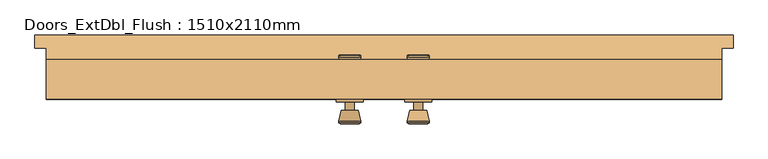
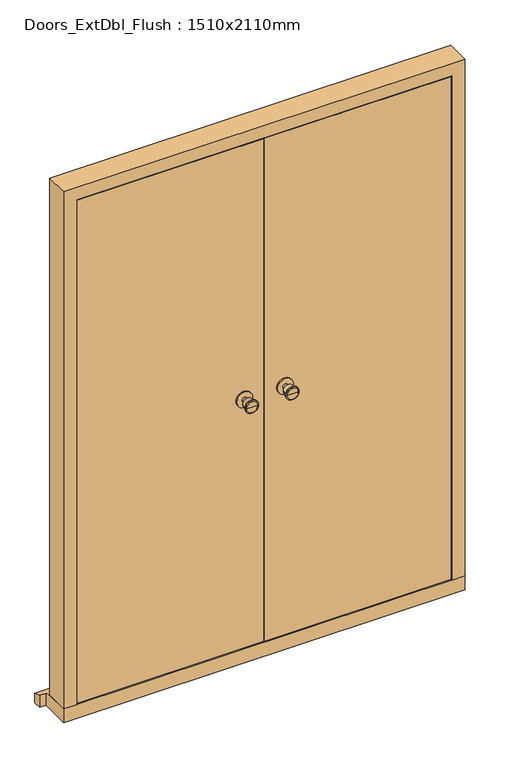
"""IFC4 building model written with IfcOpenShell, lengths in millimetres: door geometry, Doors_ExtDbl_Flush : 1510x2110mm."""

from ifc_helpers import new_model, si_unit, point, frame, frame_2d, origin, place, context, project, spatial, polyline, circle_curve, trimmed, segment, composite_curve, outline, extrude, faceted_brep, source, transform, mapped, element, save
from ifc_brep_helpers import plane_surface, cylinder_surface, revolved_surface, advanced_brep


def doors_extdbl_flush_1510x2110mm_ebd05307(model_context):
    return source(origin(), model_context, "Body", "SolidModel", [
        advanced_brep(
        [(-76.5, 108.6, 1050.0), (-66.5, 108.6, 1050.0), (-86.5, 108.6, 1050.0), (-96.9758676, 59.6, 1050.0), (-56.0241324, 59.6, 1050.0), (-76.5, 59.6, 1050.0), (-101.5, 61.4278681, 1050.0), (-51.5, 61.4278681, 1050.0), (-101.5, 64.8915463, 1050.0), (-51.5, 64.8915463, 1050.0), (-95.136236, 89.6, 1050.0), (-57.863764, 89.6, 1050.0), (-86.5, 89.6, 1050.0), (-66.5, 89.6, 1050.0)],
        [
            (0, 1),
            (1, 2, circle_curve(frame((-76.5, 108.6, 1050.0), z_axis=(0.0, 1.0, 0.0), x_axis=(1.0, 0.0, 0.0)), 10.0)),
            (2, 0),
            (2, 1, circle_curve(frame((-76.5, 108.6, 1050.0), z_axis=(0.0, 1.0, 0.0), x_axis=(1.0, 0.0, 0.0)), 10.0)),
            (3, 4, circle_curve(frame((-76.5, 59.6, 1050.0), z_axis=(0.0, -1.0, 0.0), x_axis=(1.0, 0.0, 0.0)), 20.4758676)),
            (4, 5),
            (5, 3),
            (4, 3, circle_curve(frame((-76.5, 59.6, 1050.0), z_axis=(0.0, -1.0, 0.0), x_axis=(1.0, 0.0, 0.0)), 20.4758676)),
            (6, 7, circle_curve(frame((-76.5, 61.4278681, 1050.0), z_axis=(0.0, -1.0, 0.0), x_axis=(1.0, 0.0, 0.0)), 25.0)),
            (7, 4),
            (3, 6),
            (7, 6, circle_curve(frame((-76.5, 61.4278681, 1050.0), z_axis=(0.0, -1.0, 0.0), x_axis=(1.0, 0.0, 0.0)), 25.0)),
            (8, 9, circle_curve(frame((-76.5, 64.8915463, 1050.0), z_axis=(0.0, -1.0, 0.0), x_axis=(1.0, 0.0, 0.0)), 25.0)),
            (9, 7),
            (6, 8),
            (9, 8, circle_curve(frame((-76.5, 64.8915463, 1050.0), z_axis=(0.0, -1.0, 0.0), x_axis=(1.0, 0.0, 0.0)), 25.0)),
            (10, 11, circle_curve(frame((-76.5, 89.6, 1050.0), z_axis=(0.0, -1.0, 0.0), x_axis=(1.0, 0.0, 0.0)), 18.636236)),
            (11, 9),
            (8, 10),
            (11, 10, circle_curve(frame((-76.5, 89.6, 1050.0), z_axis=(0.0, -1.0, 0.0), x_axis=(1.0, 0.0, 0.0)), 18.636236)),
            (12, 13, circle_curve(frame((-76.5, 89.6, 1050.0), z_axis=(0.0, -1.0, 0.0), x_axis=(1.0, 0.0, 0.0)), 10.0)),
            (13, 11),
            (10, 12),
            (13, 12, circle_curve(frame((-76.5, 89.6, 1050.0), z_axis=(0.0, -1.0, 0.0), x_axis=(1.0, 0.0, 0.0)), 10.0)),
            (1, 13),
            (12, 2),
        ],
        [
            plane_surface(frame((-76.5, 108.6, 1050.0), z_axis=(0.0, 1.0, 0.0), x_axis=(1.0, 0.0, 0.0))),
            plane_surface(frame((-76.5, 59.6, 1050.0), z_axis=(0.0, -1.0, 0.0), x_axis=(1.0, 0.0, 0.0))),
            revolved_surface(polyline([(-56.0241324, 59.6, 1050.0), (-51.5, 61.4278681, 1050.0)]), (-76.5, 108.6, 1050.0), (0.0, 1.0, 0.0)),
            cylinder_surface(frame((-76.5, 108.6, 1050.0), z_axis=(0.0, 1.0, 0.0), x_axis=(1.0, 0.0, 0.0)), 25.0),
            revolved_surface(polyline([(-51.5, 64.8915463, 1050.0), (-57.863764, 89.6, 1050.0)]), (-76.5, 108.6, 1050.0), (0.0, 1.0, 0.0)),
            plane_surface(frame((-76.5, 89.6, 1050.0), z_axis=(0.0, 1.0, 0.0), x_axis=(1.0, 0.0, 0.0))),
            cylinder_surface(frame((-76.5, 108.6, 1050.0), z_axis=(0.0, 1.0, 0.0), x_axis=(1.0, 0.0, 0.0)), 10.0),
        ],
        [
            (0, [[1, 2, 3]]),
            (0, [[-3, 4, -1]]),
            (1, [[5, 6, 7]]),
            (1, [[8, -7, -6]]),
            (2, [[9, 10, -5, 11]]),
            (2, [[12, -11, -8, -10]]),
            (3, [[13, 14, -9, 15]]),
            (3, [[16, -15, -12, -14]]),
            (4, [[17, 18, -13, 19]]),
            (4, [[20, -19, -16, -18]]),
            (5, [[21, 22, -17, 23]]),
            (5, [[24, -23, -20, -22]]),
            (6, [[-2, 25, -21, 26]]),
            (6, [[-4, -26, -24, -25]]),
        ],
    ),
        extrude(outline(composite_curve([segment(trimmed(circle_curve(frame_2d((1050.0, -76.5)), 30.0), [point((1050.0, -46.5))], [point((1050.0, -106.5))], False, "CARTESIAN"), True, "CONTINUOUS"), segment(trimmed(circle_curve(frame_2d((1050.0, -76.5)), 30.0), [point((1050.0, -106.5))], [point((1050.0, -46.5))], False, "CARTESIAN"), True, "CONTINUOUS")], self_intersect=False)), frame((0.0, 108.6, 0.0), z_axis=(0.0, 1.0, 0.0), x_axis=(0.0, 0.0, 1.0)), (0.0, 0.0, 1.0), 6.0),
        advanced_brep(
        [(-76.5, 164.6, 1050.0), (-86.5, 164.6, 1050.0), (-66.5, 164.6, 1050.0), (-96.9758676, 213.6, 1050.0), (-76.5, 213.6, 1050.0), (-56.0241324, 213.6, 1050.0), (-101.5, 211.7721319, 1050.0), (-51.5, 211.7721319, 1050.0), (-101.5, 208.3084537, 1050.0), (-51.5, 208.3084537, 1050.0), (-95.136236, 183.6, 1050.0), (-57.863764, 183.6, 1050.0), (-86.5, 183.6, 1050.0), (-66.5, 183.6, 1050.0)],
        [
            (0, 1),
            (1, 2, circle_curve(frame((-76.5, 164.6, 1050.0), z_axis=(0.0, -1.0, 0.0), x_axis=(1.0, 0.0, 0.0)), 10.0)),
            (2, 0),
            (2, 1, circle_curve(frame((-76.5, 164.6, 1050.0), z_axis=(0.0, -1.0, 0.0), x_axis=(1.0, 0.0, 0.0)), 10.0)),
            (3, 4),
            (4, 5),
            (5, 3, circle_curve(frame((-76.5, 213.6, 1050.0), z_axis=(0.0, 1.0, 0.0), x_axis=(1.0, 0.0, 0.0)), 20.4758676)),
            (3, 5, circle_curve(frame((-76.5, 213.6, 1050.0), z_axis=(0.0, 1.0, 0.0), x_axis=(1.0, 0.0, 0.0)), 20.4758676)),
            (6, 3),
            (5, 7),
            (7, 6, circle_curve(frame((-76.5, 211.7721319, 1050.0), z_axis=(0.0, 1.0, 0.0), x_axis=(1.0, 0.0, 0.0)), 25.0)),
            (6, 7, circle_curve(frame((-76.5, 211.7721319, 1050.0), z_axis=(0.0, 1.0, 0.0), x_axis=(1.0, 0.0, 0.0)), 25.0)),
            (8, 6),
            (7, 9),
            (9, 8, circle_curve(frame((-76.5, 208.3084537, 1050.0), z_axis=(0.0, 1.0, 0.0), x_axis=(1.0, 0.0, 0.0)), 25.0)),
            (8, 9, circle_curve(frame((-76.5, 208.3084537, 1050.0), z_axis=(0.0, 1.0, 0.0), x_axis=(1.0, 0.0, 0.0)), 25.0)),
            (10, 8),
            (9, 11),
            (11, 10, circle_curve(frame((-76.5, 183.6, 1050.0), z_axis=(0.0, 1.0, 0.0), x_axis=(1.0, 0.0, 0.0)), 18.636236)),
            (10, 11, circle_curve(frame((-76.5, 183.6, 1050.0), z_axis=(0.0, 1.0, 0.0), x_axis=(1.0, 0.0, 0.0)), 18.636236)),
            (12, 10),
            (11, 13),
            (13, 12, circle_curve(frame((-76.5, 183.6, 1050.0), z_axis=(0.0, 1.0, 0.0), x_axis=(1.0, 0.0, 0.0)), 10.0)),
            (12, 13, circle_curve(frame((-76.5, 183.6, 1050.0), z_axis=(0.0, 1.0, 0.0), x_axis=(1.0, 0.0, 0.0)), 10.0)),
            (1, 12),
            (13, 2),
        ],
        [
            plane_surface(frame((-76.5, 164.6, 1050.0), z_axis=(0.0, -1.0, 0.0), x_axis=(1.0, 0.0, 0.0))),
            plane_surface(frame((-76.5, 213.6, 1050.0), z_axis=(0.0, 1.0, 0.0), x_axis=(1.0, 0.0, 0.0))),
            revolved_surface(polyline([(-56.0241324, 213.6, 1050.0), (-51.5, 211.7721319, 1050.0)]), (-76.5, 164.6, 1050.0), (0.0, -1.0, 0.0)),
            cylinder_surface(frame((-76.5, 164.6, 1050.0), z_axis=(0.0, -1.0, 0.0), x_axis=(1.0, 0.0, 0.0)), 25.0),
            revolved_surface(polyline([(-51.5, 208.3084537, 1050.0), (-57.863764, 183.6, 1050.0)]), (-76.5, 164.6, 1050.0), (0.0, -1.0, 0.0)),
            plane_surface(frame((-76.5, 183.6, 1050.0), z_axis=(0.0, -1.0, 0.0), x_axis=(1.0, 0.0, 0.0))),
            cylinder_surface(frame((-76.5, 164.6, 1050.0), z_axis=(0.0, -1.0, 0.0), x_axis=(1.0, 0.0, 0.0)), 10.0),
        ],
        [
            (0, [[1, 2, 3]]),
            (0, [[-3, 4, -1]]),
            (1, [[5, 6, 7]]),
            (1, [[-6, -5, 8]]),
            (2, [[9, -7, 10, 11]]),
            (2, [[-10, -8, -9, 12]]),
            (3, [[13, -11, 14, 15]]),
            (3, [[-14, -12, -13, 16]]),
            (4, [[17, -15, 18, 19]]),
            (4, [[-18, -16, -17, 20]]),
            (5, [[21, -19, 22, 23]]),
            (5, [[-22, -20, -21, 24]]),
            (6, [[25, -23, 26, -2]]),
            (6, [[-26, -24, -25, -4]]),
        ],
    ),
        extrude(outline(composite_curve([segment(trimmed(circle_curve(frame_2d((1050.0, -76.5)), 30.0), [point((1050.0, -46.5))], [point((1050.0, -106.5))], False, "CARTESIAN"), True, "CONTINUOUS"), segment(trimmed(circle_curve(frame_2d((1050.0, -76.5)), 30.0), [point((1050.0, -106.5))], [point((1050.0, -46.5))], False, "CARTESIAN"), True, "CONTINUOUS")], self_intersect=False)), frame((0.0, 158.6, 0.0), z_axis=(0.0, 1.0, 0.0), x_axis=(0.0, 0.0, 1.0)), (0.0, 0.0, 1.0), 6.0),
        advanced_brep(
        [(76.5, 108.6, 1050.0), (86.5, 108.6, 1050.0), (66.5, 108.6, 1050.0), (96.9758676, 59.6, 1050.0), (76.5, 59.6, 1050.0), (56.0241324, 59.6, 1050.0), (101.5, 61.4278681, 1050.0), (51.5, 61.4278681, 1050.0), (101.5, 64.8915463, 1050.0), (51.5, 64.8915463, 1050.0), (95.136236, 89.6, 1050.0), (57.863764, 89.6, 1050.0), (86.5, 89.6, 1050.0), (66.5, 89.6, 1050.0)],
        [
            (0, 1),
            (1, 2, circle_curve(frame((76.5, 108.6, 1050.0), z_axis=(0.0, 1.0, 0.0), x_axis=(-1.0, 0.0, 0.0)), 10.0)),
            (2, 0),
            (2, 1, circle_curve(frame((76.5, 108.6, 1050.0), z_axis=(0.0, 1.0, 0.0), x_axis=(-1.0, 0.0, 0.0)), 10.0)),
            (3, 4),
            (4, 5),
            (5, 3, circle_curve(frame((76.5, 59.6, 1050.0), z_axis=(0.0, -1.0, 0.0), x_axis=(-1.0, 0.0, 0.0)), 20.4758676)),
            (3, 5, circle_curve(frame((76.5, 59.6, 1050.0), z_axis=(0.0, -1.0, 0.0), x_axis=(-1.0, 0.0, 0.0)), 20.4758676)),
            (6, 3),
            (5, 7),
            (7, 6, circle_curve(frame((76.5, 61.4278681, 1050.0), z_axis=(0.0, -1.0, 0.0), x_axis=(-1.0, 0.0, 0.0)), 25.0)),
            (6, 7, circle_curve(frame((76.5, 61.4278681, 1050.0), z_axis=(0.0, -1.0, 0.0), x_axis=(-1.0, 0.0, 0.0)), 25.0)),
            (8, 6),
            (7, 9),
            (9, 8, circle_curve(frame((76.5, 64.8915463, 1050.0), z_axis=(0.0, -1.0, 0.0), x_axis=(-1.0, 0.0, 0.0)), 25.0)),
            (8, 9, circle_curve(frame((76.5, 64.8915463, 1050.0), z_axis=(0.0, -1.0, 0.0), x_axis=(-1.0, 0.0, 0.0)), 25.0)),
            (10, 8),
            (9, 11),
            (11, 10, circle_curve(frame((76.5, 89.6, 1050.0), z_axis=(0.0, -1.0, 0.0), x_axis=(-1.0, 0.0, 0.0)), 18.636236)),
            (10, 11, circle_curve(frame((76.5, 89.6, 1050.0), z_axis=(0.0, -1.0, 0.0), x_axis=(-1.0, 0.0, 0.0)), 18.636236)),
            (12, 10),
            (11, 13),
            (13, 12, circle_curve(frame((76.5, 89.6, 1050.0), z_axis=(0.0, -1.0, 0.0), x_axis=(-1.0, 0.0, 0.0)), 10.0)),
            (12, 13, circle_curve(frame((76.5, 89.6, 1050.0), z_axis=(0.0, -1.0, 0.0), x_axis=(-1.0, 0.0, 0.0)), 10.0)),
            (1, 12),
            (13, 2),
        ],
        [
            plane_surface(frame((76.5, 108.6, 1050.0), z_axis=(0.0, 1.0, 0.0), x_axis=(-1.0, 0.0, 0.0))),
            plane_surface(frame((76.5, 59.6, 1050.0), z_axis=(0.0, -1.0, 0.0), x_axis=(-1.0, 0.0, 0.0))),
            revolved_surface(polyline([(56.0241324, 59.6, 1050.0), (51.5, 61.4278681, 1050.0)]), (76.5, 108.6, 1050.0), (0.0, 1.0, 0.0)),
            cylinder_surface(frame((76.5, 108.6, 1050.0), z_axis=(0.0, 1.0, 0.0), x_axis=(-1.0, 0.0, 0.0)), 25.0),
            revolved_surface(polyline([(51.5, 64.8915463, 1050.0), (57.863764, 89.6, 1050.0)]), (76.5, 108.6, 1050.0), (0.0, 1.0, 0.0)),
            plane_surface(frame((76.5, 89.6, 1050.0), z_axis=(0.0, 1.0, 0.0), x_axis=(-1.0, 0.0, 0.0))),
            cylinder_surface(frame((76.5, 108.6, 1050.0), z_axis=(0.0, 1.0, 0.0), x_axis=(-1.0, 0.0, 0.0)), 10.0),
        ],
        [
            (0, [[1, 2, 3]]),
            (0, [[-3, 4, -1]]),
            (1, [[5, 6, 7]]),
            (1, [[-6, -5, 8]]),
            (2, [[9, -7, 10, 11]]),
            (2, [[-10, -8, -9, 12]]),
            (3, [[13, -11, 14, 15]]),
            (3, [[-14, -12, -13, 16]]),
            (4, [[17, -15, 18, 19]]),
            (4, [[-18, -16, -17, 20]]),
            (5, [[21, -19, 22, 23]]),
            (5, [[-22, -20, -21, 24]]),
            (6, [[25, -23, 26, -2]]),
            (6, [[-26, -24, -25, -4]]),
        ],
    ),
        extrude(outline(composite_curve([segment(trimmed(circle_curve(frame_2d((1050.0, 76.5)), 30.0), [point((1050.0, 46.5))], [point((1050.0, 106.5))], False, "CARTESIAN"), True, "CONTINUOUS"), segment(trimmed(circle_curve(frame_2d((1050.0, 76.5)), 30.0), [point((1050.0, 106.5))], [point((1050.0, 46.5))], False, "CARTESIAN"), True, "CONTINUOUS")], self_intersect=False)), frame((0.0, 108.6, 0.0), z_axis=(0.0, 1.0, 0.0), x_axis=(0.0, 0.0, 1.0)), (0.0, 0.0, 1.0), 6.0),
        advanced_brep(
        [(76.5, 164.6, 1050.0), (66.5, 164.6, 1050.0), (86.5, 164.6, 1050.0), (96.9758676, 213.6, 1050.0), (56.0241324, 213.6, 1050.0), (76.5, 213.6, 1050.0), (101.5, 211.7721319, 1050.0), (51.5, 211.7721319, 1050.0), (101.5, 208.3084537, 1050.0), (51.5, 208.3084537, 1050.0), (95.136236, 183.6, 1050.0), (57.863764, 183.6, 1050.0), (86.5, 183.6, 1050.0), (66.5, 183.6, 1050.0)],
        [
            (0, 1),
            (1, 2, circle_curve(frame((76.5, 164.6, 1050.0), z_axis=(0.0, -1.0, 0.0), x_axis=(-1.0, 0.0, 0.0)), 10.0)),
            (2, 0),
            (2, 1, circle_curve(frame((76.5, 164.6, 1050.0), z_axis=(0.0, -1.0, 0.0), x_axis=(-1.0, 0.0, 0.0)), 10.0)),
            (3, 4, circle_curve(frame((76.5, 213.6, 1050.0), z_axis=(0.0, 1.0, 0.0), x_axis=(-1.0, 0.0, 0.0)), 20.4758676)),
            (4, 5),
            (5, 3),
            (4, 3, circle_curve(frame((76.5, 213.6, 1050.0), z_axis=(0.0, 1.0, 0.0), x_axis=(-1.0, 0.0, 0.0)), 20.4758676)),
            (6, 7, circle_curve(frame((76.5, 211.7721319, 1050.0), z_axis=(0.0, 1.0, 0.0), x_axis=(-1.0, 0.0, 0.0)), 25.0)),
            (7, 4),
            (3, 6),
            (7, 6, circle_curve(frame((76.5, 211.7721319, 1050.0), z_axis=(0.0, 1.0, 0.0), x_axis=(-1.0, 0.0, 0.0)), 25.0)),
            (8, 9, circle_curve(frame((76.5, 208.3084537, 1050.0), z_axis=(0.0, 1.0, 0.0), x_axis=(-1.0, 0.0, 0.0)), 25.0)),
            (9, 7),
            (6, 8),
            (9, 8, circle_curve(frame((76.5, 208.3084537, 1050.0), z_axis=(0.0, 1.0, 0.0), x_axis=(-1.0, 0.0, 0.0)), 25.0)),
            (10, 11, circle_curve(frame((76.5, 183.6, 1050.0), z_axis=(0.0, 1.0, 0.0), x_axis=(-1.0, 0.0, 0.0)), 18.636236)),
            (11, 9),
            (8, 10),
            (11, 10, circle_curve(frame((76.5, 183.6, 1050.0), z_axis=(0.0, 1.0, 0.0), x_axis=(-1.0, 0.0, 0.0)), 18.636236)),
            (12, 13, circle_curve(frame((76.5, 183.6, 1050.0), z_axis=(0.0, 1.0, 0.0), x_axis=(-1.0, 0.0, 0.0)), 10.0)),
            (13, 11),
            (10, 12),
            (13, 12, circle_curve(frame((76.5, 183.6, 1050.0), z_axis=(0.0, 1.0, 0.0), x_axis=(-1.0, 0.0, 0.0)), 10.0)),
            (1, 13),
            (12, 2),
        ],
        [
            plane_surface(frame((76.5, 164.6, 1050.0), z_axis=(0.0, -1.0, 0.0), x_axis=(-1.0, 0.0, 0.0))),
            plane_surface(frame((76.5, 213.6, 1050.0), z_axis=(0.0, 1.0, 0.0), x_axis=(-1.0, 0.0, 0.0))),
            revolved_surface(polyline([(56.0241324, 213.6, 1050.0), (51.5, 211.7721319, 1050.0)]), (76.5, 164.6, 1050.0), (0.0, -1.0, 0.0)),
            cylinder_surface(frame((76.5, 164.6, 1050.0), z_axis=(0.0, -1.0, 0.0), x_axis=(-1.0, 0.0, 0.0)), 25.0),
            revolved_surface(polyline([(51.5, 208.3084537, 1050.0), (57.863764, 183.6, 1050.0)]), (76.5, 164.6, 1050.0), (0.0, -1.0, 0.0)),
            plane_surface(frame((76.5, 183.6, 1050.0), z_axis=(0.0, -1.0, 0.0), x_axis=(-1.0, 0.0, 0.0))),
            cylinder_surface(frame((76.5, 164.6, 1050.0), z_axis=(0.0, -1.0, 0.0), x_axis=(-1.0, 0.0, 0.0)), 10.0),
        ],
        [
            (0, [[1, 2, 3]]),
            (0, [[-3, 4, -1]]),
            (1, [[5, 6, 7]]),
            (1, [[8, -7, -6]]),
            (2, [[9, 10, -5, 11]]),
            (2, [[12, -11, -8, -10]]),
            (3, [[13, 14, -9, 15]]),
            (3, [[16, -15, -12, -14]]),
            (4, [[17, 18, -13, 19]]),
            (4, [[20, -19, -16, -18]]),
            (5, [[21, 22, -17, 23]]),
            (5, [[24, -23, -20, -22]]),
            (6, [[-2, 25, -21, 26]]),
            (6, [[-4, -26, -24, -25]]),
        ],
    ),
        extrude(outline(composite_curve([segment(trimmed(circle_curve(frame_2d((1050.0, 76.5)), 30.0), [point((1050.0, 46.5))], [point((1050.0, 106.5))], False, "CARTESIAN"), True, "CONTINUOUS"), segment(trimmed(circle_curve(frame_2d((1050.0, 76.5)), 30.0), [point((1050.0, 106.5))], [point((1050.0, 46.5))], False, "CARTESIAN"), True, "CONTINUOUS")], self_intersect=False)), frame((0.0, 158.6, 0.0), z_axis=(0.0, 1.0, 0.0), x_axis=(0.0, 0.0, 1.0)), (0.0, 0.0, 1.0), 6.0),
        faceted_brep([(684.5, 203.6, 54.5), (755.0, 203.6, 54.5), (755.0, 114.6, 54.5), (706.5, 114.6, 54.5), (706.5, 161.6, 54.5), (684.5, 161.6, 54.5), (684.5, 203.6, 2039.5), (-684.5, 203.6, 2039.5), (-684.5, 203.6, 54.5), (-755.0, 203.6, 54.5), (-755.0, 203.6, 2110.0), (755.0, 203.6, 2110.0), (755.0, 114.6, 2110.0), (-755.0, 114.6, 2110.0), (-755.0, 114.6, 54.5), (-706.5, 114.6, 54.5), (-706.5, 114.6, 2061.5), (706.5, 114.6, 2061.5), (706.5, 161.6, 2061.5), (-706.5, 161.6, 2061.5), (-706.5, 161.6, 54.5), (-684.5, 161.6, 54.5), (-684.5, 161.6, 2039.5), (684.5, 161.6, 2039.5)], [[[0, 1, 2, 3, 4, 5]], [[1, 0, 6, 7, 8, 9, 10, 11]], [[2, 1, 11, 12]], [[3, 2, 12, 13, 14, 15, 16, 17]], [[4, 3, 17, 18]], [[5, 4, 18, 19, 20, 21, 22, 23]], [[0, 5, 23, 6]], [[12, 11, 10, 13]], [[18, 17, 16, 19]], [[6, 23, 22, 7]], [[8, 21, 20, 15, 14, 9]], [[13, 10, 9, 14]], [[19, 16, 15, 20]], [[7, 22, 21, 8]]]),
        faceted_brep([(780.0, 258.6, 0.0), (780.0, 258.6, 38.5947221), (780.0, 228.6, 47.2703282), (780.0, 228.6, 0.0), (-780.0, 258.6, 38.5947221), (-780.0, 258.6, 0.0), (-780.0, 228.6, 0.0), (-780.0, 228.6, 47.2703282), (755.0, 228.6, 0.0), (755.0, 114.6, 0.0), (-755.0, 114.6, 0.0), (-755.0, 228.6, 0.0), (-755.0, 228.6, 47.2703282), (-755.0, 203.6, 54.5), (755.0, 203.6, 54.5), (755.0, 228.6, 47.2703282), (-755.0, 114.6, 54.5), (755.0, 114.6, 54.5)], [[[0, 1, 2, 3]], [[4, 5, 6, 7]], [[5, 0, 3, 8, 9, 10, 11, 6]], [[1, 0, 5, 4]], [[1, 4, 7, 12, 13, 14, 15, 2]], [[13, 16, 17, 14]], [[16, 10, 9, 17]], [[12, 11, 10, 16, 13]], [[11, 12, 7, 6]], [[8, 15, 14, 17, 9]], [[15, 8, 3, 2]]]),
        extrude(outline(polyline([(703.5, 114.6), (1.5, 114.6), (1.5, 158.6), (703.5, 158.6), (703.5, 114.6)])), frame((0.0, 0.0, 58.5), z_axis=(0.0, 0.0, 1.0), x_axis=(1.0, 0.0, 0.0)), (0.0, 0.0, 1.0), 2000.0),
        extrude(outline(polyline([(-1.5, 114.6), (-703.5, 114.6), (-703.5, 158.6), (-1.5, 158.6), (-1.5, 114.6)])), frame((0.0, 0.0, 58.5), z_axis=(0.0, 0.0, 1.0), x_axis=(1.0, 0.0, 0.0)), (0.0, 0.0, 1.0), 2000.0),
    ])


if __name__ == "__main__":
    model = new_model("IFC4")
    model_context = context("Model", 3, world=origin())
    ifc_project = project(units=[si_unit("LENGTHUNIT", "METRE", prefix="MILLI")], contexts=[model_context])
    site = spatial("IfcSite", under=ifc_project)
    building = spatial("IfcBuilding", under=site)
    placement = place(None, origin())
    doors_extdbl_flush_1510x2110mm_shape = doors_extdbl_flush_1510x2110mm_ebd05307(model_context)
    element("IfcDoor", 1, ObjectType="Doors_ExtDbl_Flush : 1510x2110mm", at=placement, inside=building, context=model_context, shape_type="MappedRepresentation", body=[
        mapped(doors_extdbl_flush_1510x2110mm_shape, transform((0.0, 0.0, 0.0), x_axis=(1.0, 0.0, 0.0), y_axis=(0.0, 1.0, 0.0), z_axis=(0.0, 0.0, 1.0))),
    ])
    save(model, "model.ifc")

# Revit data of these elements
# Type "Doors_ExtDbl_Flush : 1510x2110mm"
#   Construction Type Id = "MDOOR"
#   Type Mark = "45"
#   Type Comments = "External Double"
#   Operation = "DoubleDoorSingleSwing"
#   Keynote = "L20"
#   Analytic Construction = "Metal"
#   Wrap Layers (Ext) from Ext = 0' - 4.03543"
#   Wrap Layers (Int) from Ext = 0' - 6.98819"
#   Thickness = 0' - 1.73228"
#   Rough Width = 4' - 11.44882"
#   Rough Height = 6' - 11.07087"
#   O/A Frame Width = 0' - 2.51969"
#   Heat Transfer Coefficient (U) = 3.7021 W/(m²·K)
#   Handle Z Distance = 3' - 5.33858"
#   FrameWidth = 0' - 1.65354"
#   FrameOffset - External = 0' - 0.98425"
#   FrameDepth = 0' - 3.50394"
#   Door Panel Width = 2' - 3.6378"
#   Door Panel Thickness = 0' - 1.73228"
#   Door Panel Height = 6' - 6.74016"
#   Cill Thickness = 0' - 2.14567"
#   Cill Projection = 0' - 1.1811"
#   Handle X Distance = 0' - 2.95276"
#   Height = 6' - 11.07087"
#   Structural Tolerance = 0' - 0.25591"
#   Tolerance = 0' - 0.11811"
#   Undercut = 0' - 0.15748"
#   Width = 4' - 11.44882"
#   Cill Extension = 0' - 0.98425"
#   Cavity Closer Width = 0' - 1.9685"
#   Cavity Closer Offset from Ext = 0' - 4.03543"
#   Cavity Closer Depth = 0' - 3.34646"
#   Define Thermal Properties by = 1
#   Vis - Ironmongery = yes
#   Vis - Cavity Closers = yes
#   Function = 1
#   Material Door = Door - Panel
#   Material Frame = Door - Frame/Mullion
#   Material Ironmongery = Door - Handle
#   Visual Light Transmittance = 0
#   Thermal Resistance (R) = 0
#   Solar Heat Gain Coefficient = 0
#   Wall Closure = (empty or 0)
# Element 1 (IfcDoor, "Doors_ExtDbl_Flush : 1510x2110mm")
#   Materials on its faces: "Door - Handle", "Door - Frame/Mullion", "Door - Panel"
# Materials
#   "Door - Panel": class "Wood", colour RGB 210 159 95, transparency 0, Keynote = "L20", Cost = 0
#   "Door - Frame/Mullion": class "Wood", colour RGB 212 179 113, transparency 0, Keynote = "L20", Cost = 0
#   "Door - Handle": colour RGB 0 0 0, transparency 0, Keynote = "P21", Cost = 0
